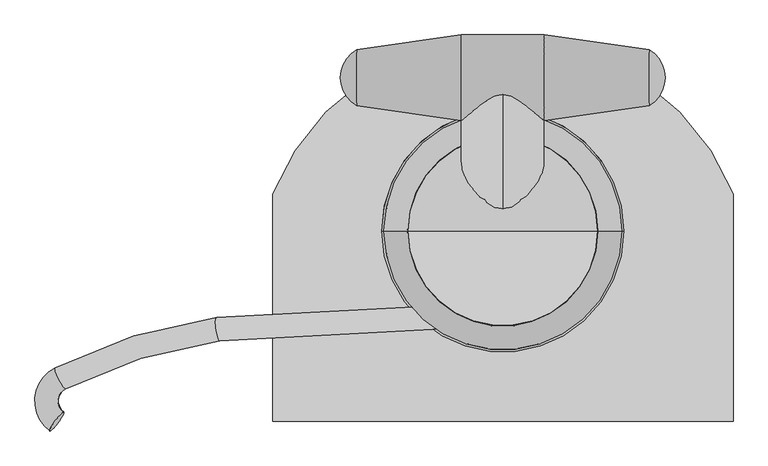
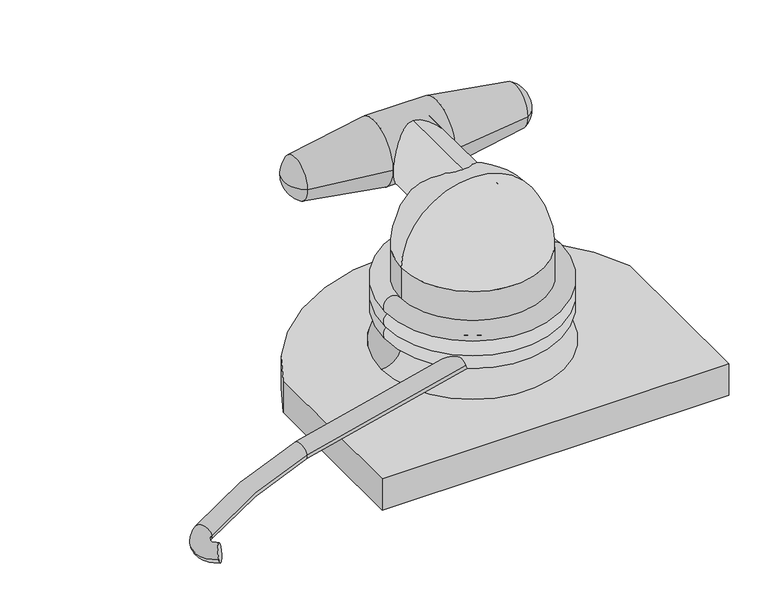
"""IFC4 building model written with IfcOpenShell, lengths in millimetres: proxy geometry."""

from ifc_helpers import new_model, si_unit, point, frame, origin, place, context, project, spatial, polyline, circle_curve, ellipse_curve, trimmed, source, transform, mapped, element, save
from ifc_brep_helpers import plane_surface, cylinder_surface, revolved_surface, advanced_brep


def generic_models_aa191242(model_context):
    return source(origin(), model_context, "Body", "AdvancedBrep", [
        advanced_brep(
        [(247.6764423, 212.4053864, 387.5), (247.6764423, 307.5946136, 387.5), (275.0, 260.0, 387.5), (70.0, 187.5, 387.5), (70.0, 332.5, 387.5), (-70.0, 187.5, 387.5), (-70.0, 332.5, 387.5), (-247.6764423, 212.4053864, 387.5), (-247.6764423, 307.5946136, 387.5), (-275.0, 260.0, 387.5)],
        [
            (0, 1, circle_curve(frame((247.6764423, 260.0, 387.5), z_axis=(1.0, 0.0, 0.0), x_axis=(0.0, 1.0, 0.0)), 47.5946136)),
            (1, 2, circle_curve(frame((219.8859464, 260.0, 387.5), z_axis=(0.0, 0.0, -1.0), x_axis=(-1.0, 0.0, 0.0)), 55.1140536)),
            (2, 0, circle_curve(frame((219.8859464, 260.0, 387.5), z_axis=(0.0, 0.0, -1.0), x_axis=(-1.0, 0.0, 0.0)), 55.1140536)),
            (1, 0, circle_curve(frame((247.6764423, 260.0, 387.5), z_axis=(1.0, 0.0, 0.0), x_axis=(0.0, 1.0, 0.0)), 47.5946136)),
            (3, 4, circle_curve(frame((70.0, 260.0, 387.5), z_axis=(1.0, 0.0, 0.0), x_axis=(0.0, 1.0, 0.0)), 72.5)),
            (4, 1),
            (0, 3),
            (4, 3, circle_curve(frame((70.0, 260.0, 387.5), z_axis=(1.0, 0.0, 0.0), x_axis=(0.0, 1.0, 0.0)), 72.5)),
            (5, 6, circle_curve(frame((-70.0, 260.0, 387.5), z_axis=(1.0, 0.0, 0.0), x_axis=(0.0, 1.0, 0.0)), 72.5)),
            (6, 4),
            (3, 5),
            (6, 5, circle_curve(frame((-70.0, 260.0, 387.5), z_axis=(1.0, 0.0, 0.0), x_axis=(0.0, 1.0, 0.0)), 72.5)),
            (7, 8, circle_curve(frame((-247.6764423, 260.0, 387.5), z_axis=(1.0, 0.0, 0.0), x_axis=(0.0, 1.0, 0.0)), 47.5946136)),
            (8, 6),
            (5, 7),
            (8, 7, circle_curve(frame((-247.6764423, 260.0, 387.5), z_axis=(1.0, 0.0, 0.0), x_axis=(0.0, 1.0, 0.0)), 47.5946136)),
            (9, 8, circle_curve(frame((-219.8859464, 260.0, 387.5), z_axis=(0.0, 0.0, -1.0), x_axis=(1.0, 0.0, 0.0)), 55.1140536)),
            (7, 9, circle_curve(frame((-219.8859464, 260.0, 387.5), z_axis=(0.0, 0.0, -1.0), x_axis=(1.0, 0.0, 0.0)), 55.1140536)),
        ],
        [
            revolved_surface(trimmed(ellipse_curve(frame((219.8859464, 260.0, 387.5), z_axis=(0.0, 0.0, 1.0), x_axis=(-1.0, 0.0, 0.0)), 55.1140536, 55.1140536), [point((275.0, 260.0, 387.5))], [point((247.6764423, 307.5946136, 387.5))], True, "CARTESIAN"), (-640.0, 260.0, 387.5), (-1.0, 0.0, 0.0)),
            revolved_surface(polyline([(247.6764423, 307.5946136, 387.5), (70.0, 332.5, 387.5)]), (-640.0, 260.0, 387.5), (-1.0, 0.0, 0.0)),
            cylinder_surface(frame((-640.0, 260.0, 387.5), z_axis=(-1.0, 0.0, 0.0), x_axis=(0.0, 1.0, 0.0)), 72.5),
            revolved_surface(polyline([(-70.0, 332.5, 387.5), (-247.6764423, 307.5946136, 387.5)]), (-640.0, 260.0, 387.5), (-1.0, 0.0, 0.0)),
            revolved_surface(trimmed(ellipse_curve(frame((-219.8859464, 260.0, 387.5), z_axis=(0.0, 0.0, 1.0), x_axis=(1.0, 0.0, 0.0)), 55.1140536, 55.1140536), [point((-247.6764423, 307.5946136, 387.5))], [point((-275.0, 260.0, 387.5))], True, "CARTESIAN"), (-640.0, 260.0, 387.5), (-1.0, 0.0, 0.0)),
        ],
        [
            (0, [[1, 2, 3]]),
            (0, [[4, -3, -2]]),
            (1, [[5, 6, -1, 7]]),
            (1, [[8, -7, -4, -6]]),
            (2, [[9, 10, -5, 11]]),
            (2, [[12, -11, -8, -10]]),
            (3, [[13, 14, -9, 15]]),
            (3, [[16, -15, -12, -14]]),
            (4, [[17, -13, 18]]),
            (4, [[-18, -16, -17]]),
        ],
    ),
        advanced_brep(
        [(-0.1765979, -2.1178376, 384.5258786), (-0.1765979, -2.1178376, 454.5258786), (-0.1765979, -2.1178376, 314.5258786), (-0.1765979, 257.8821624, 314.5258786), (-0.1765979, 257.8821624, 454.5258786), (-0.1765979, 257.8821624, 384.5258786)],
        [
            (0, 1),
            (1, 2, circle_curve(frame((-0.1765979, -2.1178376, 384.5258786), z_axis=(0.0, -1.0, 0.0), x_axis=(0.0, 0.0, 1.0)), 70.0)),
            (2, 0),
            (2, 1, circle_curve(frame((-0.1765979, -2.1178376, 384.5258786), z_axis=(0.0, -1.0, 0.0), x_axis=(0.0, 0.0, 1.0)), 70.0)),
            (3, 4, circle_curve(frame((-0.1765979, 257.8821624, 384.5258786), z_axis=(0.0, 1.0, 0.0), x_axis=(0.0, 0.0, 1.0)), 70.0)),
            (4, 5),
            (5, 3),
            (4, 3, circle_curve(frame((-0.1765979, 257.8821624, 384.5258786), z_axis=(0.0, 1.0, 0.0), x_axis=(0.0, 0.0, 1.0)), 70.0)),
            (1, 4),
            (3, 2),
        ],
        [
            plane_surface(frame((-0.1765979, -2.1178376, 384.5258786), z_axis=(0.0, -1.0, 0.0), x_axis=(0.0, 0.0, 1.0))),
            plane_surface(frame((-0.1765979, 257.8821624, 384.5258786), z_axis=(0.0, 1.0, 0.0), x_axis=(0.0, 0.0, 1.0))),
            cylinder_surface(frame((-0.1765979, 142.8821624, 384.5258786), z_axis=(0.0, -1.0, 0.0), x_axis=(0.0, 0.0, 1.0)), 70.0),
        ],
        [
            (0, [[1, 2, 3]]),
            (0, [[-3, 4, -1]]),
            (1, [[5, 6, 7]]),
            (1, [[8, -7, -6]]),
            (2, [[-2, 9, -5, 10]]),
            (2, [[-4, -10, -8, -9]]),
        ],
    ),
        advanced_brep(
        [(390.0, -322.4720769, 75.0), (390.0, 62.5279231, 75.0), (-390.0, 62.5279231, 75.0), (-390.0, -322.4720769, 75.0), (-205.0, 0.0, 75.0), (205.0, 0.0, 75.0), (390.0, -322.4720769, 0.0), (-390.0, -322.4720769, 0.0), (-390.0, 62.5279231, 0.0), (390.0, 62.5279231, 0.0), (160.0, 0.0, 300.0), (-160.0, 0.0, 300.0), (0.0, 0.0, 460.0), (160.0, 0.0, 120.0), (-160.0, 0.0, 120.0)],
        [
            (0, 1),
            (1, 2, circle_curve(frame((0.0, -91.9532089, 75.0), z_axis=(0.0, 0.0, 1.0), x_axis=(1.0, 0.0, 0.0)), 419.4811321)),
            (2, 3),
            (3, 0),
            (4, 5, circle_curve(frame((0.0, 0.0, 75.0), z_axis=(0.0, 0.0, -1.0), x_axis=(-1.0, 0.0, 0.0)), 205.0)),
            (5, 4, circle_curve(frame((0.0, 0.0, 75.0), z_axis=(0.0, 0.0, -1.0), x_axis=(-1.0, 0.0, 0.0)), 205.0)),
            (6, 7),
            (7, 8),
            (8, 9, circle_curve(frame((0.0, -91.9532089, 0.0), z_axis=(0.0, 0.0, -1.0), x_axis=(1.0, 0.0, 0.0)), 419.4811321)),
            (9, 6),
            (0, 6),
            (9, 1),
            (8, 2),
            (7, 3),
            (10, 11, circle_curve(frame((0.0, 0.0, 300.0), z_axis=(0.0, 0.0, 1.0), x_axis=(-1.0, 0.0, 0.0)), 160.0)),
            (11, 12, circle_curve(frame((0.0, 0.0, 300.0), z_axis=(0.0, 1.0, 0.0), x_axis=(1.0, 0.0, 0.0)), 160.0)),
            (12, 10, circle_curve(frame((0.0, 0.0, 300.0), z_axis=(0.0, 1.0, 0.0), x_axis=(-1.0, 0.0, 0.0)), 160.0)),
            (11, 10, circle_curve(frame((0.0, 0.0, 300.0), z_axis=(0.0, 0.0, 1.0), x_axis=(-1.0, 0.0, 0.0)), 160.0)),
            (10, 13),
            (13, 14, circle_curve(frame((0.0, 0.0, 120.0), z_axis=(0.0, 0.0, 1.0), x_axis=(-1.0, 0.0, 0.0)), 160.0)),
            (14, 11),
            (14, 13, circle_curve(frame((0.0, 0.0, 120.0), z_axis=(0.0, 0.0, 1.0), x_axis=(-1.0, 0.0, 0.0)), 160.0)),
            (13, 5, circle_curve(frame((205.0, 0.0, 120.0), z_axis=(0.0, -1.0, 0.0), x_axis=(-1.0, 0.0, 0.0)), 45.0)),
            (4, 14, circle_curve(frame((-205.0, 0.0, 120.0), z_axis=(0.0, -1.0, 0.0), x_axis=(1.0, 0.0, 0.0)), 45.0)),
        ],
        [
            plane_surface(frame((390.0, -322.4720769, 75.0), z_axis=(0.0, 0.0, 1.0), x_axis=(0.0, 1.0, 0.0))),
            plane_surface(frame((390.0, -322.4720769, 0.0), z_axis=(0.0, 0.0, -1.0), x_axis=(0.0, -1.0, 0.0))),
            plane_surface(frame((390.0, -322.4720769, 75.0), z_axis=(1.0, 0.0, 0.0), x_axis=(0.0, 0.0, -1.0))),
            cylinder_surface(frame((0.0, -91.9532089, 0.0), z_axis=(0.0, 0.0, 1.0), x_axis=(1.0, 0.0, 0.0)), 419.4811321),
            plane_surface(frame((-390.0, 62.5279231, 75.0), z_axis=(-1.0, 0.0, 0.0), x_axis=(0.0, 0.0, -1.0))),
            plane_surface(frame((-390.0, -322.4720769, 75.0), z_axis=(0.0, -1.0, 0.0), x_axis=(0.0, 0.0, -1.0))),
            revolved_surface(trimmed(ellipse_curve(frame((0.0, 0.0, 300.0), z_axis=(0.0, -1.0, 0.0), x_axis=(1.0, 0.0, 0.0)), 160.0, 160.0), [point((0.0, 0.0, 460.0))], [point((-160.0, 0.0, 300.0))], True, "CARTESIAN"), (0.0, 0.0, 380.0), (0.0, 0.0, -1.0)),
            cylinder_surface(frame((0.0, 0.0, 380.0), z_axis=(0.0, 0.0, -1.0), x_axis=(-1.0, 0.0, 0.0)), 160.0),
            revolved_surface(trimmed(ellipse_curve(frame((-205.0, 0.0, 120.0), z_axis=(0.0, 1.0, 0.0), x_axis=(1.0, 0.0, 0.0)), 45.0, 45.0), [point((-160.0, 0.0, 120.0))], [point((-205.0, 0.0, 75.0))], True, "CARTESIAN"), (0.0, 0.0, 380.0), (0.0, 0.0, -1.0)),
        ],
        [
            (0, [[1, 2, 3, 4], [5, 6]]),
            (1, [[7, 8, 9, 10]]),
            (2, [[-1, 11, -10, 12]]),
            (3, [[-2, -12, -9, 13]]),
            (4, [[-3, -13, -8, 14]]),
            (5, [[-4, -14, -7, -11]]),
            (6, [[15, 16, 17]]),
            (6, [[-16, 18, -17]]),
            (7, [[-15, 19, 20, 21]]),
            (7, [[-18, -21, 22, -19]]),
            (8, [[-20, 23, -5, 24]]),
            (8, [[-22, -24, -6, -23]]),
        ],
    ),
        advanced_brep(
        [(194.6375173, 0.0, 171.5331963), (-194.6375173, 0.0, 171.5331963), (-191.0912191, 0.0, 204.0331963), (191.0912191, 0.0, 204.0331963), (168.1800042, 0.0, 171.5331963), (-168.1800042, 0.0, 171.5331963), (171.7263024, 0.0, 204.0331963), (-171.7263024, 0.0, 204.0331963)],
        [
            (0, 1, circle_curve(frame((0.0, 0.0, 171.5331963), z_axis=(0.0, 0.0, 1.0), x_axis=(-1.0, 0.0, 0.0)), 194.6375173)),
            (1, 2, circle_curve(frame((-181.4087608, 0.0, 186.5331963), z_axis=(0.0, 1.0, 0.0), x_axis=(1.0, 0.0, 0.0)), 20.0)),
            (2, 3, circle_curve(frame((0.0, 0.0, 204.0331963), z_axis=(0.0, 0.0, -1.0), x_axis=(-1.0, 0.0, 0.0)), 191.0912191)),
            (3, 0, circle_curve(frame((181.4087608, 0.0, 186.5331963), z_axis=(0.0, 1.0, 0.0), x_axis=(-1.0, 0.0, 0.0)), 20.0)),
            (1, 0, circle_curve(frame((0.0, 0.0, 171.5331963), z_axis=(0.0, 0.0, 1.0), x_axis=(-1.0, 0.0, 0.0)), 194.6375173)),
            (3, 2, circle_curve(frame((0.0, 0.0, 204.0331963), z_axis=(0.0, 0.0, -1.0), x_axis=(-1.0, 0.0, 0.0)), 191.0912191)),
            (4, 5, circle_curve(frame((0.0, 0.0, 171.5331963), z_axis=(0.0, 0.0, 1.0), x_axis=(-1.0, 0.0, 0.0)), 168.1800042)),
            (5, 1, circle_curve(frame((-181.4087608, 0.0, 156.5331963), z_axis=(0.0, 1.0, 0.0), x_axis=(1.0, 0.0, 0.0)), 20.0)),
            (0, 4, circle_curve(frame((181.4087608, 0.0, 156.5331963), z_axis=(0.0, 1.0, 0.0), x_axis=(-1.0, 0.0, 0.0)), 20.0)),
            (5, 4, circle_curve(frame((0.0, 0.0, 171.5331963), z_axis=(0.0, 0.0, 1.0), x_axis=(-1.0, 0.0, 0.0)), 168.1800042)),
            (6, 7, circle_curve(frame((0.0, 0.0, 204.0331963), z_axis=(0.0, 0.0, 1.0), x_axis=(-1.0, 0.0, 0.0)), 171.7263024)),
            (7, 5, circle_curve(frame((-181.4087608, 0.0, 186.5331963), z_axis=(0.0, 1.0, 0.0), x_axis=(1.0, 0.0, 0.0)), 20.0)),
            (4, 6, circle_curve(frame((181.4087608, 0.0, 186.5331963), z_axis=(0.0, 1.0, 0.0), x_axis=(-1.0, 0.0, 0.0)), 20.0)),
            (7, 6, circle_curve(frame((0.0, 0.0, 204.0331963), z_axis=(0.0, 0.0, 1.0), x_axis=(-1.0, 0.0, 0.0)), 171.7263024)),
            (2, 7, circle_curve(frame((-181.4087608, 0.0, 221.5331963), z_axis=(0.0, 1.0, 0.0), x_axis=(1.0, 0.0, 0.0)), 20.0)),
            (6, 3, circle_curve(frame((181.4087608, 0.0, 221.5331963), z_axis=(0.0, 1.0, 0.0), x_axis=(-1.0, 0.0, 0.0)), 20.0)),
        ],
        [
            revolved_surface(trimmed(ellipse_curve(frame((-181.4087608, 0.0, 186.5331963), z_axis=(0.0, -1.0, 0.0), x_axis=(1.0, 0.0, 0.0)), 20.0, 20.0), [point((-191.0912191, 0.0, 204.0331963))], [point((-194.6375173, 0.0, 171.5331963))], True, "CARTESIAN"), (0.0, 0.0, 75.0), (0.0, 0.0, -1.0)),
            revolved_surface(trimmed(ellipse_curve(frame((-181.4087608, 0.0, 156.5331963), z_axis=(0.0, -1.0, 0.0), x_axis=(1.0, 0.0, 0.0)), 20.0, 20.0), [point((-194.6375173, 0.0, 171.5331963))], [point((-168.1800042, 0.0, 171.5331963))], True, "CARTESIAN"), (0.0, 0.0, 75.0), (0.0, 0.0, -1.0)),
            revolved_surface(trimmed(ellipse_curve(frame((-181.4087608, 0.0, 186.5331963), z_axis=(0.0, -1.0, 0.0), x_axis=(1.0, 0.0, 0.0)), 20.0, 20.0), [point((-168.1800042, 0.0, 171.5331963))], [point((-171.7263024, 0.0, 204.0331963))], True, "CARTESIAN"), (0.0, 0.0, 75.0), (0.0, 0.0, -1.0)),
            revolved_surface(trimmed(ellipse_curve(frame((-181.4087608, 0.0, 221.5331963), z_axis=(0.0, -1.0, 0.0), x_axis=(1.0, 0.0, 0.0)), 20.0, 20.0), [point((-171.7263024, 0.0, 204.0331963))], [point((-191.0912191, 0.0, 204.0331963))], True, "CARTESIAN"), (0.0, 0.0, 75.0), (0.0, 0.0, -1.0)),
        ],
        [
            (0, [[1, 2, 3, 4]]),
            (0, [[5, -4, 6, -2]]),
            (1, [[7, 8, -1, 9]]),
            (1, [[10, -9, -5, -8]]),
            (2, [[11, 12, -7, 13]]),
            (2, [[14, -13, -10, -12]]),
            (3, [[-3, 15, -11, 16]]),
            (3, [[-6, -16, -14, -15]]),
        ],
    ),
        advanced_brep(
        [(-101.8465406, -126.1177797, 154.2240967), (-103.0260544, -166.0997279, 153.9948225), (-479.4497919, -186.1964943, 80.82546), (-484.7253112, -146.5591718, 79.8000029), (-740.4482144, -267.4852227, 30.092506), (-757.8322882, -231.6191453, 26.7133843), (-767.06714, -339.149621, 24.918311), (-743.8335176, -306.9036429, 29.4344697)],
        [
            (0, 1, circle_curve(frame((-102.4362975, -146.1087538, 154.1094596), z_axis=(0.9811841795550622, -0.03003976123504567, 0.19072288414293861), x_axis=(-0.029487846212598274, -0.999548704538674, -0.00573185666260996)), 20.0)),
            (1, 0, circle_curve(frame((-102.4362975, -146.1087538, 154.1094596), z_axis=(0.9811841795550622, -0.03003976123504567, 0.19072288414293861), x_axis=(-0.029487846212598274, -0.999548704538674, -0.00573185666260996)), 20.0)),
            (2, 1, circle_curve(frame((-171.8091264, -2497.6376079, 140.6247477), z_axis=(0.19080899537653223, 0.0, -0.9816271834476664), x_axis=(0.02948784621259624, 0.9995487045386741, 0.005731856662609566)), 2332.5905675)),
            (0, 3, circle_curve(frame((-171.8091264, -2497.6376079, 140.6247477), z_axis=(-0.19080899537653223, 0.0, 0.9816271834476664), x_axis=(0.02948784621259624, 0.9995487045386741, 0.005731856662609566)), 2372.5905675)),
            (3, 2, circle_curve(frame((-482.0875516, -166.377833, 80.3127315), z_axis=(0.9727268307067922, 0.13435649032646466, 0.18907894205932646), x_axis=(0.13188798317708111, -0.9909330620718811, 0.02563642694150949)), 20.0)),
            (2, 3, circle_curve(frame((-482.0875516, -166.377833, 80.3127315), z_axis=(0.9727268307067922, 0.1343564903264646, 0.18907894205932646), x_axis=(0.13188798317708106, -0.9909330620718811, 0.025636426941509482)), 20.0)),
            (4, 2, circle_curve(frame((-365.7366138, -1040.5741644, 102.9290627), z_axis=(0.19080899537653223, 0.0, -0.9816271834476664), x_axis=(-0.13188798317708333, 0.9909330620718808, -0.025636426941509922)), 862.1951399)),
            (3, 5, circle_curve(frame((-365.7366138, -1040.5741644, 102.9290627), z_axis=(-0.19080899537653223, 0.0, 0.9816271834476664), x_axis=(-0.13188798317708333, 0.9909330620718808, -0.025636426941509922)), 902.1951399)),
            (5, 4, circle_curve(frame((-749.1402513, -249.552184, 28.4029452), z_axis=(0.880177914734015, 0.44273615752785767, 0.17108925516217857), x_axis=(0.43460184732451324, -0.8966519362704058, 0.08447804143475662)), 20.0)),
            (4, 5, circle_curve(frame((-749.1402513, -249.552184, 28.4029452), z_axis=(0.880177914734015, 0.44273615752785767, 0.17108925516217857), x_axis=(0.43460184732451324, -0.8966519362704058, 0.08447804143475662)), 20.0)),
            (6, 7, circle_curve(frame((-755.4503288, -323.0266319, 27.1763903), z_axis=(0.7913382156615573, -0.5917119752071984, 0.1538205669927736), x_axis=(0.5808405596348976, 0.8061494516504961, 0.11290396754154913)), 20.0)),
            (7, 6, circle_curve(frame((-755.4503288, -323.0266319, 27.1763903), z_axis=(0.7913382156615573, -0.5917119752071984, 0.1538205669927736), x_axis=(0.5808405596348976, 0.8061494516504961, 0.11290396754154913)), 20.0)),
            (7, 4, circle_curve(frame((-730.3875471, -288.241961, 32.0481016), z_axis=(0.19080899537653223, 0.0, -0.9816271834476664), x_axis=(-0.4346018473245169, 0.8966519362704041, -0.08447804143475734)), 23.1491591)),
            (5, 6, circle_curve(frame((-730.3875471, -288.241961, 32.0481016), z_axis=(-0.19080899537653223, 0.0, 0.9816271834476664), x_axis=(-0.4346018473245169, 0.8966519362704041, -0.08447804143475734)), 63.1491591)),
        ],
        [
            plane_surface(frame((-102.8461054, -160.0, 154.029801), z_axis=(0.9811841795550624, -0.030039761235043594, 0.19072288414293861), x_axis=(-0.1908089953765322, 0.0, 0.9816271834476665))),
            revolved_surface(trimmed(ellipse_curve(frame((-102.4362975, -146.1087538, 154.1094596), z_axis=(0.9811841795550622, -0.03003976123504567, 0.19072288414293861), x_axis=(-0.029487846212598274, -0.999548704538674, -0.00573185666260996)), 20.0, 20.0), [point((-101.8465406, -126.1177797, 154.2240967))], [point((-103.0260544, -166.0997279, 153.9948225))], True, "CARTESIAN"), (-171.8091264, -2497.6376079, 140.6247477), (-0.19080899537653223, 0.0, 0.9816271834476664)),
            revolved_surface(trimmed(ellipse_curve(frame((-102.4362975, -146.1087538, 154.1094596), z_axis=(0.9811841795550622, -0.03003976123504567, 0.19072288414293861), x_axis=(-0.029487846212598274, -0.999548704538674, -0.00573185666260996)), 20.0, 20.0), [point((-103.0260544, -166.0997279, 153.9948225))], [point((-101.8465406, -126.1177797, 154.2240967))], True, "CARTESIAN"), (-171.8091264, -2497.6376079, 140.6247477), (-0.19080899537653223, 0.0, 0.9816271834476664)),
            revolved_surface(trimmed(ellipse_curve(frame((-482.0875516, -166.377833, 80.3127315), z_axis=(0.9727268307067922, 0.134356490326465, 0.18907894205932652), x_axis=(0.13188798317708145, -0.990933062071881, 0.02563642694150954)), 20.0, 20.0), [point((-484.7253112, -146.5591718, 79.8000029))], [point((-479.4497919, -186.1964943, 80.82546))], True, "CARTESIAN"), (-365.7366138, -1040.5741644, 102.9290627), (-0.19080899537653223, 0.0, 0.9816271834476664)),
            revolved_surface(trimmed(ellipse_curve(frame((-482.0875516, -166.377833, 80.3127315), z_axis=(0.9727268307067922, 0.134356490326465, 0.18907894205932652), x_axis=(0.13188798317708145, -0.990933062071881, 0.02563642694150954)), 20.0, 20.0), [point((-479.4497919, -186.1964943, 80.82546))], [point((-484.7253112, -146.5591718, 79.8000029))], True, "CARTESIAN"), (-365.7366138, -1040.5741644, 102.9290627), (-0.19080899537653223, 0.0, 0.9816271834476664)),
            plane_surface(frame((-747.3780866, -311.8231554, 28.7454753), z_axis=(0.7913382156615587, -0.5917119752071969, 0.1538205669927738), x_axis=(-0.19080899537653223, 0.0, 0.9816271834476665))),
            revolved_surface(trimmed(ellipse_curve(frame((-749.1402513, -249.552184, 28.4029452), z_axis=(0.8801779147340141, 0.44273615752785955, 0.1710892551621783), x_axis=(0.4346018473245151, -0.896651936270405, 0.08447804143475703)), 20.0, 20.0), [point((-757.8322882, -231.6191453, 26.7133843))], [point((-740.4482144, -267.4852227, 30.092506))], True, "CARTESIAN"), (-730.3875471, -288.241961, 32.0481016), (-0.19080899537653223, 0.0, 0.9816271834476664)),
            revolved_surface(trimmed(ellipse_curve(frame((-749.1402513, -249.552184, 28.4029452), z_axis=(0.8801779147340141, 0.44273615752785955, 0.1710892551621783), x_axis=(0.4346018473245151, -0.896651936270405, 0.08447804143475703)), 20.0, 20.0), [point((-740.4482144, -267.4852227, 30.092506))], [point((-757.8322882, -231.6191453, 26.7133843))], True, "CARTESIAN"), (-730.3875471, -288.241961, 32.0481016), (-0.19080899537653223, 0.0, 0.9816271834476664)),
        ],
        [
            (0, [[1, 2]]),
            (1, [[3, -1, 4, 5]]),
            (2, [[-4, -2, -3, 6]]),
            (3, [[7, -5, 8, 9]]),
            (4, [[-8, -6, -7, 10]]),
            (5, [[11, 12]]),
            (6, [[13, -9, 14, -12]]),
            (7, [[-14, -10, -13, -11]]),
        ],
    ),
    ])


if __name__ == "__main__":
    model = new_model("IFC4")
    model_context = context("Model", 3, world=origin())
    ifc_project = project(units=[si_unit("LENGTHUNIT", "METRE", prefix="MILLI")], contexts=[model_context])
    site = spatial("IfcSite", under=ifc_project)
    building = spatial("IfcBuilding", under=site)
    placement = place(None, origin())
    generic_models_shape = generic_models_aa191242(model_context)
    element("IfcBuildingElementProxy", 1, Name="Generic Models", at=placement, inside=building, context=model_context, shape_type="MappedRepresentation", body=[
        mapped(generic_models_shape, transform((0.0, 0.0, 0.0), x_axis=(1.0, 0.0, 0.0), y_axis=(0.0, 1.0, 0.0), z_axis=(0.0, 0.0, 1.0))),
    ])
    save(model, "model.ifc")

# Revit data of these elements
# Type
#   Rope Hide [instance] = yes
#   Rope [instance] = Rope
#   Bollard = Bollard
#   Default Elevation = 0
# Element 1 (IfcBuildingElementProxy)
#   Materials on its faces: "Bollard", "Rope"
# Materials
#   "Rope": class "Generic", colour RGB 192 128 68, transparency 0, Cost = 0
#   "Bollard": class "Generic", colour RGB 226 219 42, transparency 0, Cost = 0
